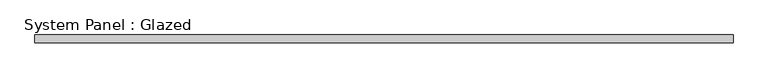
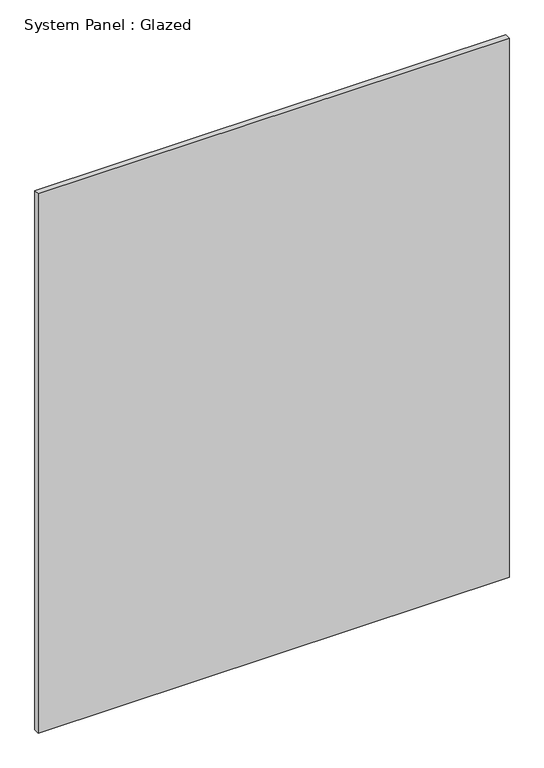
"""IFC4 building model written with IfcOpenShell, lengths in millimetres: plate geometry, System Panel : Glazed."""

from ifc_helpers import new_model, si_unit, origin, origin_with_axes, place, context, project, spatial, polyline, outline, extrude, source, transform, mapped, element, save


def system_panel_glazed_45dfe0f7(model_context):
    return source(origin(), model_context, "Body", "SweptSolid", [
        extrude(outline(polyline([(1107.2228829, 19.05), (-1107.2228829, 19.05), (-1107.2228829, 44.45), (1107.2228829, 44.45), (1107.2228829, 19.05)])), origin_with_axes(), (0.0, 0.0, 1.0), 2679.7),
    ])


if __name__ == "__main__":
    model = new_model("IFC4")
    model_context = context("Model", 3, world=origin())
    ifc_project = project(units=[si_unit("LENGTHUNIT", "METRE", prefix="MILLI")], contexts=[model_context])
    site = spatial("IfcSite", under=ifc_project)
    building = spatial("IfcBuilding", under=site)
    placement = place(None, origin())
    system_panel_glazed_shape = system_panel_glazed_45dfe0f7(model_context)
    element("IfcPlate", 1, ObjectType="System Panel : Glazed", at=placement, inside=building, context=model_context, shape_type="MappedRepresentation", body=[
        mapped(system_panel_glazed_shape, transform((0.0, 0.0, 0.0), x_axis=(1.0, 0.0, 0.0), y_axis=(0.0, 1.0, 0.0), z_axis=(0.0, 0.0, 1.0))),
    ])
    save(model, "model.ifc")

# Revit data of these elements
# Type "System Panel : Glazed"
#   Construction Type Id = "GSP4R"
#   Analytic Construction = "1/8 in Pilkington single glazing"
#   Visual Light Transmittance = 0.9
#   Solar Heat Gain Coefficient = 0.86
#   Heat Transfer Coefficient (U) = 1.18115 BTU/(h·ft²·°F)
#   Define Thermal Properties by = 1
# Element 1 (IfcPlate, "System Panel : Glazed")
#   Materials on its faces: "Glass"
# Materials
#   "Glass": class "Glass", colour RGB 0 128 192, transparency 0.75, Description = "Soda Lime Glass", Cost = 0
